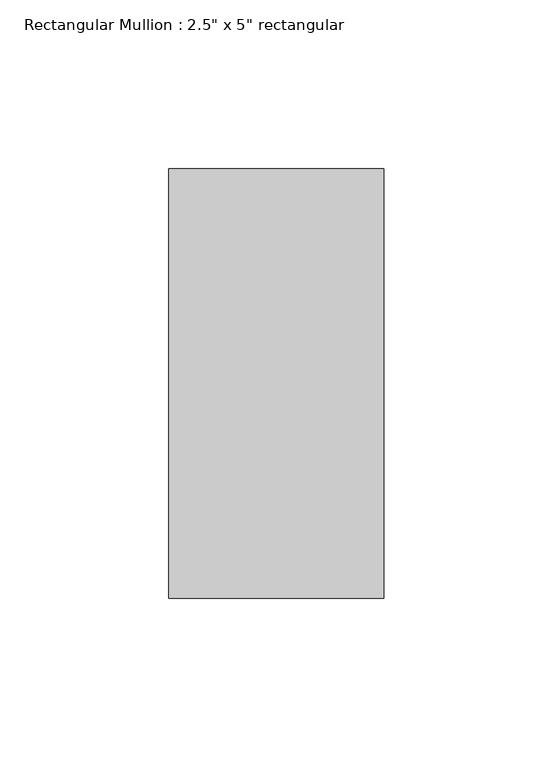
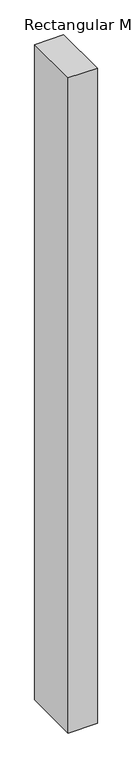
"""IFC4 building model written with IfcOpenShell, lengths in millimetres: member geometry."""

from ifc_helpers import new_model, si_unit, frame, origin, place, context, project, spatial, polyline, outline, extrude, source, transform, mapped, element, save


def member_d4c304d5(model_context):
    return source(origin(), model_context, "Body", "SweptSolid", [
        extrude(outline(polyline([(0.0, 63.5), (0.0, -63.5), (-63.5, -63.5), (-63.5, 63.5), (0.0, 63.5)])), frame((0.0, 0.0, -1513.5761917), z_axis=(0.0, 0.0, 1.0), x_axis=(1.0, 0.0, 0.0)), (0.0, 0.0, 1.0), 1513.5761917),
    ])


if __name__ == "__main__":
    model = new_model("IFC4")
    model_context = context("Model", 3, world=origin())
    ifc_project = project(units=[si_unit("LENGTHUNIT", "METRE", prefix="MILLI")], contexts=[model_context])
    site = spatial("IfcSite", under=ifc_project)
    building = spatial("IfcBuilding", under=site)
    placement = place(None, origin())
    member_shape = member_d4c304d5(model_context)
    element("IfcMember", 1, ObjectType="Rectangular Mullion : 2.5\" x 5\" rectangular", at=placement, inside=building, context=model_context, shape_type="MappedRepresentation", body=[
        mapped(member_shape, transform((0.0, 0.0, 0.0), x_axis=(1.0, 0.0, 0.0), y_axis=(0.0, 1.0, 0.0), z_axis=(0.0, 0.0, 1.0))),
    ])
    save(model, "model.ifc")

# Revit data of these elements
# Type "Rectangular Mullion : 2.5\" x 5\" rectangular"
#   built-in parameter 1007304 = 0.416667 (stored number, unit not read)
#   built-in parameter 1007301 = 0.104167 (stored number, unit not read)
#   built-in parameter 1007300 = 0.104167 (stored number, unit not read)
# Element 1 (IfcMember, "Rectangular Mullion : 2.5\" x 5\" rectangular")
#   Materials on its faces: "Aluminum"
# Materials
#   "Aluminum": class "Metal", colour RGB 247 247 247, transparency 0, Description = "Aluminum 6061", Cost = 0
